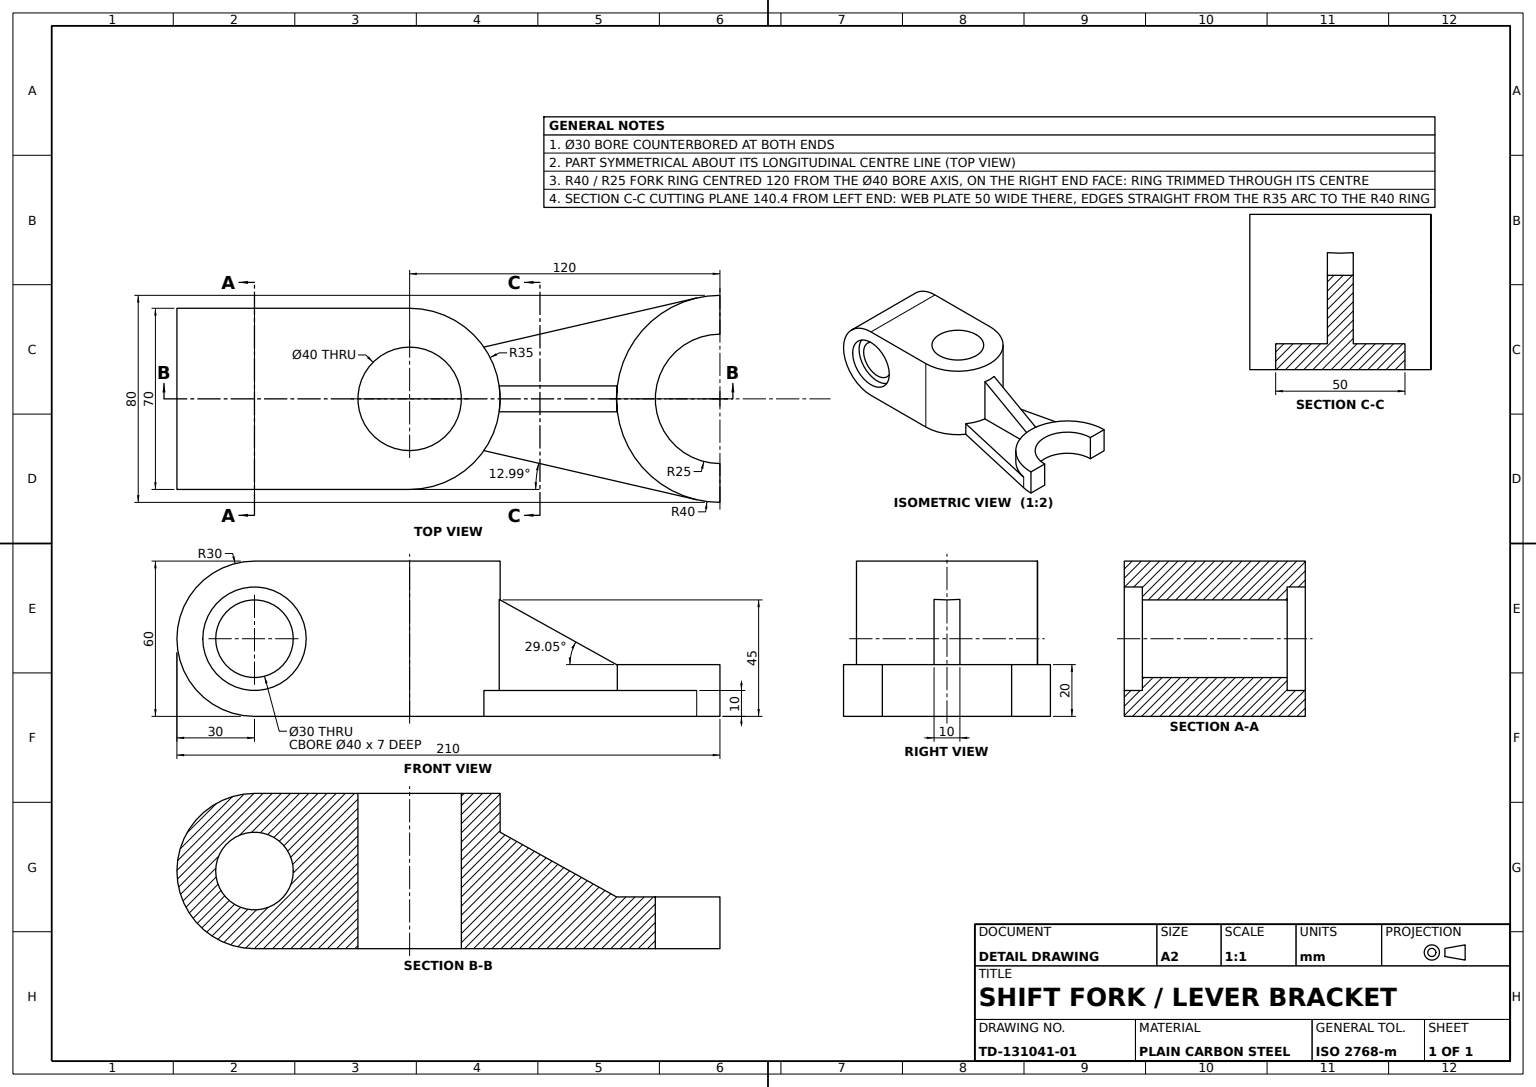
from build123d import *

# Parameters (mm, degrees)
BASE_BLOCK_DEPTH              = 60
BLOCK_SIDE_PROFILE_CUT_DEPTH  = 129.840987267
VERTICAL_BORE_SKETCH_R        = 20
VERTICAL_BORE_40_DEPTH        = 114.688170009
HORIZONTAL_BORE_SKETCH_R      = 15
HORIZONTAL_BORE_30_DEPTH      = 129.840987267
COUNTERBORE_SIDE_A_SKETCH_R   = 20
COUNTERBORE_SIDE_A_40X7_DEPTH = 7
COUNTERBORE_START             = -7
COUNTERBORE_SIDE_B_SKETCH_R   = 20
COUNTERBORE_SIDE_B_40X7_DEPTH = 7
FORK_ARM_DEPTH                = 20
ARM_WEB_PLATE_DEPTH           = 10
ARM_RIB_REACH                 = 142
ARM_RIB_SKETCH_WALL_W         = 333.478150704
ARM_RIB_SKETCH_WALL_H         = 10


with BuildPart() as part:
    # Base Block Sketch → Base Block (new body)
    with BuildSketch(Plane(origin=(0, 0, 0), x_dir=(1, 0, 0), z_dir=(0, 1, 0))):
        with BuildLine():
            Line((0, 35), (-90, 35))
            Line((-90, 35), (-90, -35))
            Line((-90, -35), (0, -35))
            ThreePointArc((0, -35), (35, 0), (0, 35))
        make_face()
    extrude(amount=BASE_BLOCK_DEPTH)

    # Block Side Profile Sketch → Block Side Profile Cut (cut, through all)
    with BuildSketch(Plane.XY.offset(35)):
        with BuildLine():
            Line((-60, 60), (-120, 60))
            Line((-120, 60), (-120, 0))
            Line((-120, 0), (-60, 0))
            ThreePointArc((-60, 0), (-90, 30), (-60, 60))
        make_face()
    extrude(amount=-BLOCK_SIDE_PROFILE_CUT_DEPTH, mode=Mode.SUBTRACT)

    # Vertical Bore Sketch → Vertical Bore Ø40 (cut, through all)
    with BuildSketch(Plane(origin=(0, 60, 0), x_dir=(1, 0, 0), z_dir=(0, 1, 0))):
        with Locations(Location((0, 0, 0), (0, 0, 270))):
            Circle(VERTICAL_BORE_SKETCH_R)
    extrude(amount=-VERTICAL_BORE_40_DEPTH, mode=Mode.SUBTRACT)

    # Horizontal Bore Sketch → Horizontal Bore Ø30 (cut, through all)
    with BuildSketch(Plane.XY.offset(35)):
        with Locations((-60, 30)):
            Circle(HORIZONTAL_BORE_SKETCH_R)
    extrude(amount=-HORIZONTAL_BORE_30_DEPTH, mode=Mode.SUBTRACT)

    # Counterbore Side A Sketch → Counterbore Side A Ø40x7 (cut)
    with BuildSketch(Plane.XY.offset(35)):
        with Locations((-60, 30)):
            Circle(COUNTERBORE_SIDE_A_SKETCH_R)
    extrude(amount=-COUNTERBORE_SIDE_A_40X7_DEPTH, mode=Mode.SUBTRACT)

    # Counterbore Side B Sketch → Counterbore Side B Ø40x7 (cut)
    with BuildSketch(Plane(origin=(0, 0, -35), x_dir=(-1, 0, 0), z_dir=(0, 0, -1)).offset(COUNTERBORE_START)):
        with Locations(Location((60, 30, 0), (0, 0, 180))):
            Circle(COUNTERBORE_SIDE_B_SKETCH_R)
    extrude(amount=COUNTERBORE_SIDE_B_40X7_DEPTH, mode=Mode.SUBTRACT)



with BuildPart() as body_2:
    # Fork Arm Sketch → Fork Arm (new body)
    with BuildSketch(Plane(origin=(0, 0, 0), x_dir=(1, 0, 0), z_dir=(0, 1, 0))):
        with BuildLine():
            Line((120, 40), (120, 25))
            ThreePointArc((120, 25), (95, 0), (120, -25))
            Line((120, -25), (120, -40))
            ThreePointArc((120, -40), (80, 0), (120, 40))
        make_face()
    extrude(amount=FORK_ARM_DEPTH)


with BuildPart() as part_1:
    add(part.part)

    add(body_2.part)  # Arm Web Plate merges body 2
    # Arm Web Plate Sketch → Arm Web Plate (add)
    with BuildSketch(Plane(origin=(0, 0, 0), x_dir=(1, 0, 0), z_dir=(0, 1, 0))):
        with BuildLine():
            Line((111.011327845, 38.976964644), (28.722813233, 20))
            ThreePointArc((28.722813233, 20), (35, 0), (28.722813233, -20))
            Line((28.722813233, -20), (111.011327845, -38.976964644))
            ThreePointArc((111.011327845, -38.976964644), (80, 0), (111.011327845, 38.976964644))
        make_face()
    extrude(amount=ARM_WEB_PLATE_DEPTH)

    # Arm Rib Sketch wall → Arm Rib (add, up to next)
    with BuildSketch(Plane(origin=(57.5, 32.5, 0), x_dir=(0.874157276122, -0.485642931179, 0), z_dir=(0.485642931179, 0.874157276122, 0)), mode=Mode.PRIVATE) as arm_rib_sk1:
        Rectangle(ARM_RIB_SKETCH_WALL_W, ARM_RIB_SKETCH_WALL_H)
    arm_rib_tool1 = extrude(arm_rib_sk1.sketch, amount=-ARM_RIB_REACH, mode=Mode.PRIVATE) - part_1.part
    add(arm_rib_tool1.solids().sort_by_distance((57.5, 32.5, 0))[0])


solid = part_1.part
